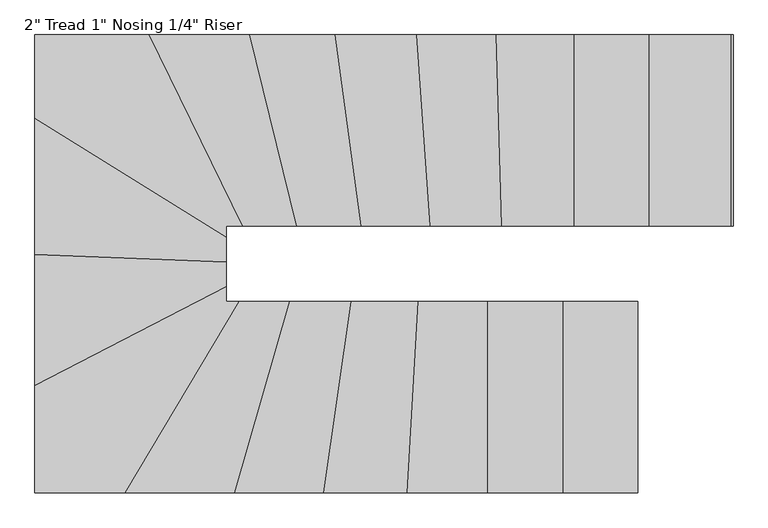
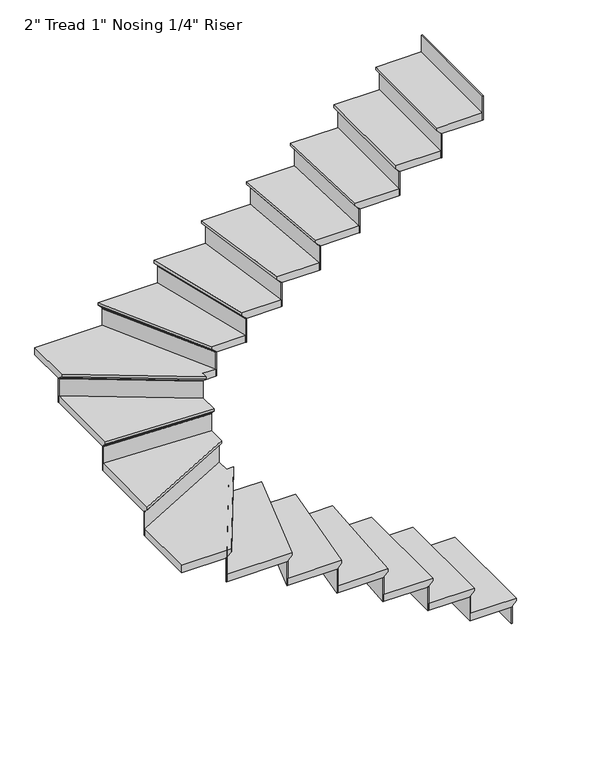
"""IFC4 building model written with IfcOpenShell, lengths in millimetres: stair flight geometry."""

from ifc_helpers import new_model, si_unit, origin, place, context, project, spatial, faceted_brep, source, transform, mapped, element, save


def stair_flight_bf45dea3(model_context):
    return source(origin(), model_context, "Body", "Brep", [
        faceted_brep([(-6703.8653968, -267.5702467, 150.2833333), (-6703.8653968, -267.5702467, 169.3333333), (-6703.8653968, -978.7702467, 169.3333333), (-6703.8653968, -978.7702467, 150.2833333), (-6729.2653968, -267.5702467, 124.8833333), (-6729.2653968, -978.7702467, 124.8833333), (-7008.6653968, -267.5702467, 169.3333333), (-7008.6653968, -978.7702467, 169.3333333), (-6729.2653968, -978.7702467, 118.5333333), (-7008.6653968, -978.7702467, 118.5333333), (-7008.6653968, -267.5702467, 118.5333333), (-6729.2653968, -267.5702467, 118.5333333)], [[[0, 1, 2, 3]], [[4, 0, 3, 5]], [[2, 1, 6, 7]], [[8, 9, 10, 11]], [[2, 7, 9, 8, 5, 3]], [[8, 11, 4, 5]], [[6, 1, 0, 4, 11, 10]], [[7, 6, 10, 9]]]),
        faceted_brep([(-6729.2653968, -267.5702467, 118.5333333), (-6729.2653968, -267.5702467, 0.0), (-6735.6153968, -267.5702467, 0.0), (-6735.6153968, -267.5702467, 118.5333333), (-6729.2653968, -978.7702467, 118.5333333), (-6735.6153968, -978.7702467, 118.5333333), (-6735.6153968, -978.7702467, 0.0), (-6729.2653968, -978.7702467, 0.0)], [[[0, 1, 2, 3]], [[4, 5, 6, 7]], [[1, 0, 4, 7]], [[2, 1, 7, 6]], [[3, 2, 6, 5]], [[0, 3, 5, 4]]]),
        faceted_brep([(-7008.6653968, -267.5702467, 287.8666667), (-7008.6653968, -267.5702467, 118.5333333), (-7015.0153968, -267.5702467, 118.5333333), (-7015.0153968, -267.5702467, 287.8666667), (-7008.6653968, -978.7702467, 287.8666667), (-7015.0153968, -978.7702467, 287.8666667), (-7015.0153968, -978.7702467, 118.5333333), (-7008.6653968, -978.7702467, 118.5333333)], [[[0, 1, 2, 3]], [[4, 5, 6, 7]], [[1, 0, 4, 7]], [[2, 1, 7, 6]], [[3, 2, 6, 5]], [[0, 3, 5, 4]]]),
        faceted_brep([(-6983.2653968, -978.7702467, 338.6666667), (-6983.2653968, -267.5702467, 338.6666667), (-7288.0653968, -267.5702467, 338.6666667), (-7288.0653968, -978.7702467, 338.6666667), (-7008.6653968, -978.7702467, 287.8666667), (-7288.0653968, -978.7702467, 287.8666667), (-7288.0653968, -267.5702467, 287.8666667), (-7008.6653968, -267.5702467, 287.8666667), (-7008.6653968, -978.7702467, 294.2166667), (-6983.2653968, -978.7702467, 319.6166667), (-7008.6653968, -267.5702467, 294.2166667), (-6983.2653968, -267.5702467, 319.6166667)], [[[0, 1, 2, 3]], [[4, 5, 6, 7]], [[0, 3, 5, 4, 8, 9]], [[4, 7, 10, 8]], [[2, 1, 11, 10, 7, 6]], [[3, 2, 6, 5]], [[11, 1, 0, 9]], [[10, 11, 9, 8]]]),
        faceted_brep([(-7288.0653968, -267.5702467, 457.2), (-7288.0653968, -267.5702467, 287.8666667), (-7294.4153968, -267.5702467, 287.8666667), (-7294.4153968, -267.5702467, 457.2), (-7288.0653968, -978.7702467, 457.2), (-7294.4153968, -978.7702467, 457.2), (-7294.4153968, -978.7702467, 287.8666667), (-7288.0653968, -978.7702467, 287.8666667)], [[[0, 1, 2, 3]], [[4, 5, 6, 7]], [[1, 0, 4, 7]], [[2, 1, 7, 6]], [[3, 2, 6, 5]], [[0, 3, 5, 4]]]),
        faceted_brep([(-7262.6653968, -978.7702467, 508.0), (-7262.6653968, -267.5702467, 508.0), (-7547.2244303, -267.5702467, 508.0), (-7587.7889272, -978.7702467, 508.0), (-7288.0653968, -978.7702467, 457.2), (-7587.7889272, -978.7702467, 457.2), (-7547.2244303, -267.5702467, 457.2), (-7288.0653968, -267.5702467, 457.2), (-7288.0653968, -978.7702467, 463.55), (-7262.6653968, -978.7702467, 488.95), (-7288.0653968, -267.5702467, 463.55), (-7262.6653968, -267.5702467, 488.95)], [[[0, 1, 2, 3]], [[4, 5, 6, 7]], [[0, 3, 5, 4, 8, 9]], [[4, 7, 10, 8]], [[2, 1, 11, 10, 7, 6]], [[3, 2, 6, 5]], [[11, 1, 0, 9]], [[10, 11, 9, 8]]]),
        faceted_brep([(-7547.2244303, -267.5702467, 626.5333333), (-7547.2244303, -267.5702467, 457.2), (-7553.5847508, -267.5702467, 457.2), (-7553.5847508, -267.5702467, 626.5333333), (-7587.7889272, -978.7702467, 626.5333333), (-7594.1492476, -978.7702467, 626.5333333), (-7594.1492476, -978.7702467, 457.2), (-7587.7889272, -978.7702467, 457.2)], [[[0, 1, 2, 3]], [[4, 5, 6, 7]], [[1, 0, 4, 7]], [[2, 1, 7, 6]], [[3, 2, 6, 5]], [[0, 3, 5, 4]]]),
        faceted_brep([(-7562.3476453, -978.7702467, 677.3333333), (-7521.7831484, -267.5702467, 677.3333333), (-7796.1994529, -267.5702467, 677.3333333), (-7898.0496202, -978.7702467, 677.3333333), (-7587.7889272, -978.7702467, 626.5333333), (-7898.0496202, -978.7702467, 626.5333333), (-7796.1994529, -267.5702467, 626.5333333), (-7547.2244303, -267.5702467, 626.5333333), (-7587.7889272, -978.7702467, 632.8833333), (-7562.3476453, -978.7702467, 658.2833333), (-7547.2244303, -267.5702467, 632.8833333), (-7521.7831484, -267.5702467, 658.2833333)], [[[0, 1, 2, 3]], [[4, 5, 6, 7]], [[0, 3, 5, 4, 8, 9]], [[4, 7, 10, 8]], [[2, 1, 11, 10, 7, 6]], [[3, 2, 6, 5]], [[11, 1, 0, 9]], [[10, 11, 9, 8]]]),
        faceted_brep([(-7796.1994529, -267.5702467, 795.8666667), (-7796.1994529, -267.5702467, 626.5333333), (-7802.6142378, -267.5702467, 626.5333333), (-7802.6142378, -267.5702467, 795.8666667), (-7898.0496202, -978.7702467, 795.8666667), (-7904.4644051, -978.7702467, 795.8666667), (-7904.4644051, -978.7702467, 626.5333333), (-7898.0496202, -978.7702467, 626.5333333)], [[[0, 1, 2, 3]], [[4, 5, 6, 7]], [[1, 0, 4, 7]], [[2, 1, 7, 6]], [[3, 2, 6, 5]], [[0, 3, 5, 4]]]),
        faceted_brep([(-7872.3904805, -978.7702467, 846.6666667), (-7770.5403132, -267.5702467, 846.6666667), (-8024.7111002, -267.5702467, 846.6666667), (-8229.8915277, -978.7702467, 846.6666667), (-7898.0496202, -978.7702467, 795.8666667), (-8229.8915277, -978.7702467, 795.8666667), (-8024.7111002, -267.5702467, 795.8666667), (-7796.1994529, -267.5702467, 795.8666667), (-7898.0496202, -978.7702467, 802.2166667), (-7872.3904805, -978.7702467, 827.6166667), (-7796.1994529, -267.5702467, 802.2166667), (-7770.5403132, -267.5702467, 827.6166667)], [[[0, 1, 2, 3]], [[4, 5, 6, 7]], [[0, 3, 5, 4, 8, 9]], [[4, 7, 10, 8]], [[2, 1, 11, 10, 7, 6]], [[3, 2, 6, 5]], [[11, 1, 0, 9]], [[10, 11, 9, 8]]]),
        faceted_brep([(-8024.7111002, -267.5702467, 965.2), (-8024.7111002, -267.5702467, 795.8666667), (-8031.3200795, -267.5702467, 795.8666667), (-8031.3200795, -267.5702467, 965.2), (-8229.8915277, -978.7702467, 965.2), (-8236.500507, -978.7702467, 965.2), (-8236.500507, -978.7702467, 795.8666667), (-8229.8915277, -978.7702467, 795.8666667)], [[[0, 1, 2, 3]], [[4, 5, 6, 7]], [[1, 0, 4, 7]], [[2, 1, 7, 6]], [[3, 2, 6, 5]], [[0, 3, 5, 4]]]),
        faceted_brep([(-8203.4556106, -978.7702467, 1016.0), (-7998.2751831, -267.5702467, 1016.0), (-8215.4900718, -267.5702467, 1016.0), (-8638.2587821, -978.7702467, 1016.0), (-8229.8915277, -978.7702467, 965.2), (-8638.2587821, -978.7702467, 965.2), (-8215.4900718, -267.5702467, 965.2), (-8024.7111002, -267.5702467, 965.2), (-8229.8915277, -978.7702467, 971.55), (-8203.4556106, -978.7702467, 996.95), (-8024.7111002, -267.5702467, 971.55), (-7998.2751831, -267.5702467, 996.95)], [[[0, 1, 2, 3]], [[4, 5, 6, 7]], [[0, 3, 5, 4, 8, 9]], [[4, 7, 10, 8]], [[2, 1, 11, 10, 7, 6]], [[3, 2, 6, 5]], [[11, 1, 0, 9]], [[10, 11, 9, 8]]]),
        faceted_brep([(-8215.4900718, -267.5702467, 1134.5333333), (-8215.4900718, -267.5702467, 965.2), (-8222.8772915, -267.5702467, 965.2), (-8222.8772915, -267.5702467, 1134.5333333), (-8638.2587821, -978.7702467, 1134.5333333), (-8645.6460018, -978.7702467, 1134.5333333), (-8645.6460018, -978.7702467, 965.2), (-8638.2587821, -978.7702467, 965.2)], [[[0, 1, 2, 3]], [[4, 5, 6, 7]], [[1, 0, 4, 7]], [[2, 1, 7, 6]], [[3, 2, 6, 5]], [[0, 3, 5, 4]]]),
        faceted_brep([(-8942.7970887, -550.9609034, 1185.3333333), (-8942.7970887, -978.7702467, 1185.3333333), (-8608.709903, -978.7702467, 1185.3333333), (-8185.9411927, -267.5702467, 1185.3333333), (-8231.5970887, -267.5702467, 1185.3333333), (-8231.5970887, -183.3035044, 1185.3333333), (-8942.7970887, -978.7702467, 1134.5333333), (-8942.7970887, -550.9609034, 1134.5333333), (-8231.5970887, -183.3035044, 1134.5333333), (-8231.5970887, -267.5702467, 1134.5333333), (-8215.4900718, -267.5702467, 1134.5333333), (-8638.2587821, -978.7702467, 1134.5333333), (-8638.2587821, -978.7702467, 1140.8833333), (-8608.709903, -978.7702467, 1166.2833333), (-8215.4900718, -267.5702467, 1140.8833333), (-8185.9411927, -267.5702467, 1166.2833333)], [[[0, 1, 2, 3, 4, 5]], [[6, 7, 8, 9, 10, 11]], [[1, 0, 7, 6]], [[2, 1, 6, 11, 12, 13]], [[11, 10, 14, 12]], [[4, 3, 15, 14, 10, 9]], [[5, 4, 9, 8]], [[0, 5, 8, 7]], [[15, 3, 2, 13]], [[14, 15, 13, 12]]]),
        faceted_brep([(-8231.5970887, -183.3035044, 1303.8666667), (-8231.5970887, -183.3035044, 1134.5333333), (-8231.5970887, -176.1551951, 1134.5333333), (-8231.5970887, -176.1551951, 1303.8666667), (-8942.7970887, -550.9609034, 1303.8666667), (-8942.7970887, -543.8125941, 1303.8666667), (-8942.7970887, -543.8125941, 1134.5333333), (-8942.7970887, -550.9609034, 1134.5333333)], [[[0, 1, 2, 3]], [[4, 5, 6, 7]], [[1, 0, 4, 7]], [[2, 1, 7, 6]], [[3, 2, 6, 5]], [[0, 3, 5, 4]]]),
        faceted_brep([(-8942.7970887, -579.5541407, 1354.6666667), (-8231.5970887, -211.8967417, 1354.6666667), (-8231.5970887, -94.9288835, 1354.6666667), (-8942.7970887, -67.5761944, 1354.6666667), (-8942.7970887, -550.9609034, 1303.8666667), (-8942.7970887, -67.5761944, 1303.8666667), (-8231.5970887, -94.9288835, 1303.8666667), (-8231.5970887, -183.3035044, 1303.8666667), (-8942.7970887, -550.9609034, 1310.2166667), (-8942.7970887, -579.5541407, 1335.6166667), (-8231.5970887, -183.3035044, 1310.2166667), (-8231.5970887, -211.8967417, 1335.6166667)], [[[0, 1, 2, 3]], [[4, 5, 6, 7]], [[0, 3, 5, 4, 8, 9]], [[4, 7, 10, 8]], [[3, 2, 6, 5]], [[11, 1, 0, 9]], [[10, 11, 9, 8]], [[2, 1, 11, 10, 7, 6]]]),
        faceted_brep([(-8231.5970887, -94.9288835, 1473.2), (-8231.5970887, -94.9288835, 1303.8666667), (-8231.5970887, -88.5741889, 1303.8666667), (-8231.5970887, -88.5741889, 1473.2), (-8942.7970887, -67.5761944, 1473.2), (-8942.7970887, -61.2214998, 1473.2), (-8942.7970887, -61.2214998, 1303.8666667), (-8942.7970887, -67.5761944, 1303.8666667)], [[[0, 1, 2, 3]], [[4, 5, 6, 7]], [[1, 0, 4, 7]], [[2, 1, 7, 6]], [[3, 2, 6, 5]], [[0, 3, 5, 4]]]),
        faceted_brep([(-8942.7970887, -92.9949729, 1524.0), (-8231.5970887, -120.3476619, 1524.0), (-8231.5970887, 2.6376943, 1524.0), (-8942.7970887, 443.8067684, 1524.0), (-8942.7970887, -67.5761944, 1473.2), (-8942.7970887, 443.8067684, 1473.2), (-8231.5970887, 2.6376943, 1473.2), (-8231.5970887, -94.9288835, 1473.2), (-8942.7970887, -67.5761944, 1479.55), (-8942.7970887, -92.9949729, 1504.95), (-8231.5970887, -94.9288835, 1479.55), (-8231.5970887, -120.3476619, 1504.95)], [[[0, 1, 2, 3]], [[4, 5, 6, 7]], [[0, 3, 5, 4, 8, 9]], [[4, 7, 10, 8]], [[2, 1, 11, 10, 7, 6]], [[3, 2, 6, 5]], [[11, 1, 0, 9]], [[10, 11, 9, 8]]]),
        faceted_brep([(-8231.5970887, 2.6376943, 1642.5333333), (-8231.5970887, 2.6376943, 1473.2), (-8231.5970887, 10.110197, 1473.2), (-8231.5970887, 10.110197, 1642.5333333), (-8942.7970887, 443.8067684, 1642.5333333), (-8942.7970887, 451.2792711, 1642.5333333), (-8942.7970887, 451.2792711, 1473.2), (-8942.7970887, 443.8067684, 1473.2)], [[[0, 1, 2, 3]], [[4, 5, 6, 7]], [[1, 0, 4, 7]], [[2, 1, 7, 6]], [[3, 2, 6, 5]], [[0, 3, 5, 4]]]),
        faceted_brep([(-8490.7794443, 723.0297533, 1693.3333333), (-8942.7970887, 723.0297533, 1693.3333333), (-8942.7970887, 413.9167576, 1693.3333333), (-8231.5970887, -27.2523165, 1693.3333333), (-8231.5970887, 11.8297533, 1693.3333333), (-8142.8507291, 11.8297533, 1693.3333333), (-8942.7970887, 723.0297533, 1642.5333333), (-8490.7794443, 723.0297533, 1642.5333333), (-8142.8507291, 11.8297533, 1642.5333333), (-8231.5970887, 11.8297533, 1642.5333333), (-8231.5970887, 2.6376943, 1642.5333333), (-8942.7970887, 443.8067684, 1642.5333333), (-8231.5970887, 2.6376943, 1648.8833333), (-8942.7970887, 443.8067684, 1648.8833333), (-8231.5970887, -27.2523165, 1674.2833333), (-8942.7970887, 413.9167576, 1674.2833333)], [[[0, 1, 2, 3, 4, 5]], [[6, 7, 8, 9, 10, 11]], [[1, 0, 7, 6]], [[11, 10, 12, 13]], [[4, 3, 14, 12, 10, 9]], [[5, 4, 9, 8]], [[0, 5, 8, 7]], [[14, 3, 2, 15]], [[12, 14, 15, 13]], [[2, 1, 6, 11, 13, 15]]]),
        faceted_brep([(-8142.8507291, 11.8297533, 1811.8666667), (-8142.8507291, 11.8297533, 1642.5333333), (-8135.7815791, 11.8297533, 1642.5333333), (-8135.7815791, 11.8297533, 1811.8666667), (-8490.7794443, 723.0297533, 1811.8666667), (-8483.7102943, 723.0297533, 1811.8666667), (-8483.7102943, 723.0297533, 1642.5333333), (-8490.7794443, 723.0297533, 1642.5333333)], [[[0, 1, 2, 3]], [[4, 5, 6, 7]], [[1, 0, 4, 7]], [[2, 1, 7, 6]], [[3, 2, 6, 5]], [[0, 3, 5, 4]]]),
        faceted_brep([(-8519.0560444, 723.0297533, 1862.6666667), (-8171.1273292, 11.8297533, 1862.6666667), (-7944.72112, 11.8297533, 1862.6666667), (-8119.5650514, 723.0297533, 1862.6666667), (-8490.7794443, 723.0297533, 1811.8666667), (-8119.5650514, 723.0297533, 1811.8666667), (-7944.72112, 11.8297533, 1811.8666667), (-8142.8507291, 11.8297533, 1811.8666667), (-8490.7794443, 723.0297533, 1818.2166667), (-8519.0560444, 723.0297533, 1843.6166667), (-8142.8507291, 11.8297533, 1818.2166667), (-8171.1273292, 11.8297533, 1843.6166667)], [[[0, 1, 2, 3]], [[4, 5, 6, 7]], [[0, 3, 5, 4, 8, 9]], [[4, 7, 10, 8]], [[2, 1, 11, 10, 7, 6]], [[3, 2, 6, 5]], [[11, 1, 0, 9]], [[10, 11, 9, 8]]]),
        faceted_brep([(-7944.72112, 11.8297533, 1981.2), (-7944.72112, 11.8297533, 1811.8666667), (-7938.1820411, 11.8297533, 1811.8666667), (-7938.1820411, 11.8297533, 1981.2), (-8119.5650514, 723.0297533, 1981.2), (-8113.0259724, 723.0297533, 1981.2), (-8113.0259724, 723.0297533, 1811.8666667), (-8119.5650514, 723.0297533, 1811.8666667)], [[[0, 1, 2, 3]], [[4, 5, 6, 7]], [[1, 0, 4, 7]], [[2, 1, 7, 6]], [[3, 2, 6, 5]], [[0, 3, 5, 4]]]),
        faceted_brep([(-8145.7213672, 723.0297533, 2032.0), (-7970.8774359, 11.8297533, 2032.0), (-7705.3592628, 11.8297533, 2032.0), (-7801.1805362, 723.0297533, 2032.0), (-8119.5650514, 723.0297533, 1981.2), (-7801.1805362, 723.0297533, 1981.2), (-7705.3592628, 11.8297533, 1981.2), (-7944.72112, 11.8297533, 1981.2), (-8119.5650514, 723.0297533, 1987.55), (-8145.7213672, 723.0297533, 2012.95), (-7944.72112, 11.8297533, 1987.55), (-7970.8774359, 11.8297533, 2012.95)], [[[0, 1, 2, 3]], [[4, 5, 6, 7]], [[0, 3, 5, 4, 8, 9]], [[4, 7, 10, 8]], [[2, 1, 11, 10, 7, 6]], [[3, 2, 6, 5]], [[11, 1, 0, 9]], [[10, 11, 9, 8]]]),
        faceted_brep([(-7705.3592628, 11.8297533, 2150.5333333), (-7705.3592628, 11.8297533, 1981.2), (-7698.9518873, 11.8297533, 1981.2), (-7698.9518873, 11.8297533, 2150.5333333), (-7801.1805362, 723.0297533, 2150.5333333), (-7794.7731607, 723.0297533, 2150.5333333), (-7794.7731607, 723.0297533, 1981.2), (-7801.1805362, 723.0297533, 1981.2)], [[[0, 1, 2, 3]], [[4, 5, 6, 7]], [[1, 0, 4, 7]], [[2, 1, 7, 6]], [[3, 2, 6, 5]], [[0, 3, 5, 4]]]),
        faceted_brep([(-7826.8100382, 723.0297533, 2201.3333333), (-7730.9887648, 11.8297533, 2201.3333333), (-7448.8717052, 11.8297533, 2201.3333333), (-7499.20006, 723.0297533, 2201.3333333), (-7801.1805362, 723.0297533, 2150.5333333), (-7499.20006, 723.0297533, 2150.5333333), (-7448.8717052, 11.8297533, 2150.5333333), (-7705.3592628, 11.8297533, 2150.5333333), (-7801.1805362, 723.0297533, 2156.8833333), (-7826.8100382, 723.0297533, 2182.2833333), (-7705.3592628, 11.8297533, 2156.8833333), (-7730.9887648, 11.8297533, 2182.2833333)], [[[0, 1, 2, 3]], [[4, 5, 6, 7]], [[0, 3, 5, 4, 8, 9]], [[4, 7, 10, 8]], [[2, 1, 11, 10, 7, 6]], [[3, 2, 6, 5]], [[11, 1, 0, 9]], [[10, 11, 9, 8]]]),
        faceted_brep([(-7448.8717052, 11.8297533, 2319.8666667), (-7448.8717052, 11.8297533, 2150.5333333), (-7442.5058255, 11.8297533, 2150.5333333), (-7442.5058255, 11.8297533, 2319.8666667), (-7499.20006, 723.0297533, 2319.8666667), (-7492.8341803, 723.0297533, 2319.8666667), (-7492.8341803, 723.0297533, 2150.5333333), (-7499.20006, 723.0297533, 2150.5333333)], [[[0, 1, 2, 3]], [[4, 5, 6, 7]], [[1, 0, 4, 7]], [[2, 1, 7, 6]], [[3, 2, 6, 5]], [[0, 3, 5, 4]]]),
        faceted_brep([(-7524.6635789, 723.0297533, 2370.6666667), (-7474.3352241, 11.8297533, 2370.6666667), (-7184.3086292, 11.8297533, 2370.6666667), (-7205.0685363, 723.0297533, 2370.6666667), (-7499.20006, 723.0297533, 2319.8666667), (-7205.0685363, 723.0297533, 2319.8666667), (-7184.3086292, 11.8297533, 2319.8666667), (-7448.8717052, 11.8297533, 2319.8666667), (-7499.20006, 723.0297533, 2326.2166667), (-7524.6635789, 723.0297533, 2351.6166667), (-7448.8717052, 11.8297533, 2326.2166667), (-7474.3352241, 11.8297533, 2351.6166667)], [[[0, 1, 2, 3]], [[4, 5, 6, 7]], [[0, 3, 5, 4, 8, 9]], [[4, 7, 10, 8]], [[2, 1, 11, 10, 7, 6]], [[3, 2, 6, 5]], [[11, 1, 0, 9]], [[10, 11, 9, 8]]]),
        faceted_brep([(-7184.3086292, 11.8297533, 2489.2), (-7184.3086292, 11.8297533, 2319.8666667), (-7177.9559245, 11.8297533, 2319.8666667), (-7177.9559245, 11.8297533, 2489.2), (-7205.0685363, 723.0297533, 2489.2), (-7198.7158316, 723.0297533, 2489.2), (-7198.7158316, 723.0297533, 2319.8666667), (-7205.0685363, 723.0297533, 2319.8666667)], [[[0, 1, 2, 3]], [[4, 5, 6, 7]], [[1, 0, 4, 7]], [[2, 1, 7, 6]], [[3, 2, 6, 5]], [[0, 3, 5, 4]]]),
        faceted_brep([(-7230.4793551, 723.0297533, 2540.0), (-7209.7194479, 11.8297533, 2540.0), (-6915.2994015, 11.8297533, 2540.0), (-6915.2994015, 723.0297533, 2540.0), (-7205.0685363, 723.0297533, 2489.2), (-6915.2994015, 723.0297533, 2489.2), (-6915.2994015, 11.8297533, 2489.2), (-7184.3086292, 11.8297533, 2489.2), (-7205.0685363, 723.0297533, 2495.55), (-7230.4793551, 723.0297533, 2520.95), (-7184.3086292, 11.8297533, 2495.55), (-7209.7194479, 11.8297533, 2520.95)], [[[0, 1, 2, 3]], [[4, 5, 6, 7]], [[0, 3, 5, 4, 8, 9]], [[4, 7, 10, 8]], [[2, 1, 11, 10, 7, 6]], [[3, 2, 6, 5]], [[11, 1, 0, 9]], [[10, 11, 9, 8]]]),
        faceted_brep([(-6915.2994015, 11.8297533, 2658.5333333), (-6915.2994015, 11.8297533, 2489.2), (-6908.9494015, 11.8297533, 2489.2), (-6908.9494015, 11.8297533, 2658.5333333), (-6915.2994015, 723.0297533, 2658.5333333), (-6908.9494015, 723.0297533, 2658.5333333), (-6908.9494015, 723.0297533, 2489.2), (-6915.2994015, 723.0297533, 2489.2)], [[[0, 1, 2, 3]], [[4, 5, 6, 7]], [[1, 0, 4, 7]], [[2, 1, 7, 6]], [[3, 2, 6, 5]], [[0, 3, 5, 4]]]),
        faceted_brep([(-6940.6994015, 723.0297533, 2709.3333333), (-6940.6994015, 11.8297533, 2709.3333333), (-6635.8994015, 11.8297533, 2709.3333333), (-6635.8994015, 723.0297533, 2709.3333333), (-6915.2994015, 723.0297533, 2658.5333333), (-6635.8994015, 723.0297533, 2658.5333333), (-6635.8994015, 11.8297533, 2658.5333333), (-6915.2994015, 11.8297533, 2658.5333333), (-6915.2994015, 723.0297533, 2664.8833333), (-6940.6994015, 723.0297533, 2690.2833333), (-6915.2994015, 11.8297533, 2664.8833333), (-6940.6994015, 11.8297533, 2690.2833333)], [[[0, 1, 2, 3]], [[4, 5, 6, 7]], [[0, 3, 5, 4, 8, 9]], [[4, 7, 10, 8]], [[2, 1, 11, 10, 7, 6]], [[3, 2, 6, 5]], [[11, 1, 0, 9]], [[10, 11, 9, 8]]]),
        faceted_brep([(-6635.8994015, 11.8297533, 2827.8666667), (-6635.8994015, 11.8297533, 2658.5333333), (-6629.5494015, 11.8297533, 2658.5333333), (-6629.5494015, 11.8297533, 2827.8666667), (-6635.8994015, 723.0297533, 2827.8666667), (-6629.5494015, 723.0297533, 2827.8666667), (-6629.5494015, 723.0297533, 2658.5333333), (-6635.8994015, 723.0297533, 2658.5333333)], [[[0, 1, 2, 3]], [[4, 5, 6, 7]], [[1, 0, 4, 7]], [[2, 1, 7, 6]], [[3, 2, 6, 5]], [[0, 3, 5, 4]]]),
        faceted_brep([(-6356.4994015, 11.8297533, 2997.2), (-6356.4994015, 11.8297533, 2827.8666667), (-6350.1494015, 11.8297533, 2827.8666667), (-6350.1494015, 11.8297533, 2997.2), (-6356.4994015, 723.0297533, 2997.2), (-6350.1494015, 723.0297533, 2997.2), (-6350.1494015, 723.0297533, 2827.8666667), (-6356.4994015, 723.0297533, 2827.8666667)], [[[0, 1, 2, 3]], [[4, 5, 6, 7]], [[1, 0, 4, 7]], [[2, 1, 7, 6]], [[3, 2, 6, 5]], [[0, 3, 5, 4]]]),
        faceted_brep([(-6661.2994015, 723.0297533, 2878.6666667), (-6661.2994015, 11.8297533, 2878.6666667), (-6356.4994015, 11.8297533, 2878.6666667), (-6356.4994015, 723.0297533, 2878.6666667), (-6635.8994015, 723.0297533, 2827.8666667), (-6356.4994015, 723.0297533, 2827.8666667), (-6356.4994015, 11.8297533, 2827.8666667), (-6635.8994015, 11.8297533, 2827.8666667), (-6635.8994015, 723.0297533, 2834.2166667), (-6661.2994015, 723.0297533, 2859.6166667), (-6635.8994015, 11.8297533, 2834.2166667), (-6661.2994015, 11.8297533, 2859.6166667)], [[[0, 1, 2, 3]], [[4, 5, 6, 7]], [[0, 3, 5, 4, 8, 9]], [[4, 7, 10, 8]], [[2, 1, 11, 10, 7, 6]], [[3, 2, 6, 5]], [[11, 1, 0, 9]], [[10, 11, 9, 8]]]),
    ])


if __name__ == "__main__":
    model = new_model("IFC4")
    model_context = context("Model", 3, world=origin())
    ifc_project = project(units=[si_unit("LENGTHUNIT", "METRE", prefix="MILLI")], contexts=[model_context])
    site = spatial("IfcSite", under=ifc_project)
    building = spatial("IfcBuilding", under=site)
    placement = place(None, origin())
    stair_flight_shape = stair_flight_bf45dea3(model_context)
    element("IfcStairFlight", 1, ObjectType="2\" Tread 1\" Nosing 1/4\" Riser", at=placement, inside=building, context=model_context, shape_type="MappedRepresentation", body=[
        mapped(stair_flight_shape, transform((0.0, 0.0, 0.0), x_axis=(1.0, 0.0, 0.0), y_axis=(0.0, 1.0, 0.0), z_axis=(0.0, 0.0, 1.0))),
    ])
    save(model, "model.ifc")
